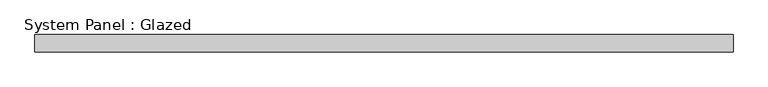
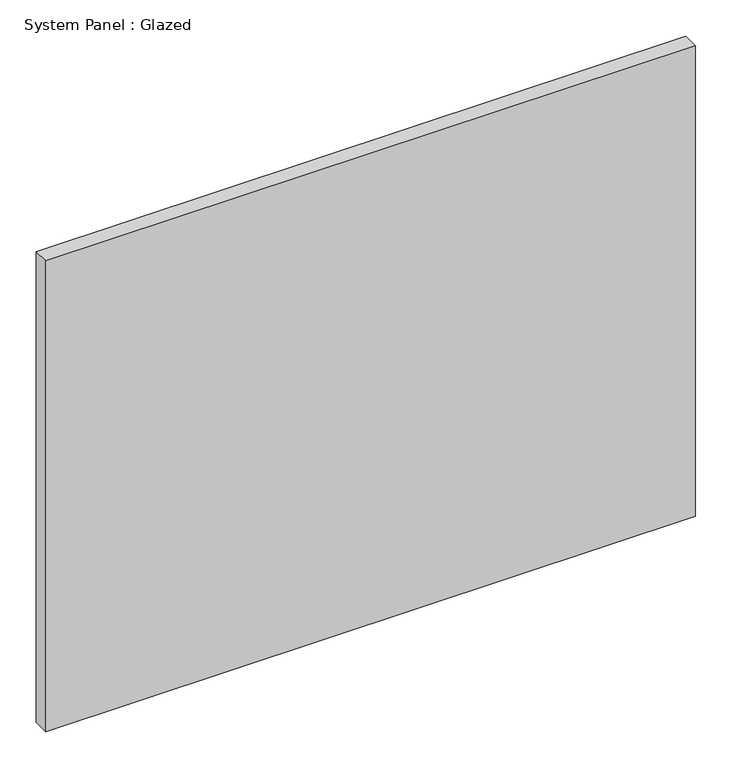
"""IFC4 building model written with IfcOpenShell, lengths in millimetres: plate geometry, System Panel : Glazed."""

from ifc_helpers import new_model, si_unit, origin, origin_with_axes, place, context, project, spatial, polyline, outline, extrude, source, transform, mapped, element, save


def system_panel_glazed_d348d9e0(model_context):
    return source(origin(), model_context, "Body", "SweptSolid", [
        extrude(outline(polyline([(514.35, 19.05), (-514.35, 19.05), (-514.35, 44.45), (514.35, 44.45), (514.35, 19.05)])), origin_with_axes(), (0.0, 0.0, 1.0), 787.4),
    ])


if __name__ == "__main__":
    model = new_model("IFC4")
    model_context = context("Model", 3, world=origin())
    ifc_project = project(units=[si_unit("LENGTHUNIT", "METRE", prefix="MILLI")], contexts=[model_context])
    site = spatial("IfcSite", under=ifc_project)
    building = spatial("IfcBuilding", under=site)
    placement = place(None, origin())
    system_panel_glazed_shape = system_panel_glazed_d348d9e0(model_context)
    element("IfcPlate", 1, ObjectType="System Panel : Glazed", at=placement, inside=building, context=model_context, shape_type="MappedRepresentation", body=[
        mapped(system_panel_glazed_shape, transform((0.0, 0.0, 0.0), x_axis=(1.0, 0.0, 0.0), y_axis=(0.0, 1.0, 0.0), z_axis=(0.0, 0.0, 1.0))),
    ])
    save(model, "model.ifc")

# Revit data of these elements
# Type "System Panel : Glazed"
#   Construction Type Id = "GSP4R"
#   Analytic Construction = "1/8 in Pilkington single glazing"
#   Visual Light Transmittance = 0.9
#   Solar Heat Gain Coefficient = 0.86
#   Heat Transfer Coefficient (U) = 1.18115 BTU/(h·ft²·°F)
# Element 1 (IfcPlate, "System Panel : Glazed")
#   Materials on its faces: "Glass"
# Materials
#   "Glass": class "Glass", colour RGB 0 128 192, transparency 0.75, Description = "Soda Lime Glass", Cost = 0
